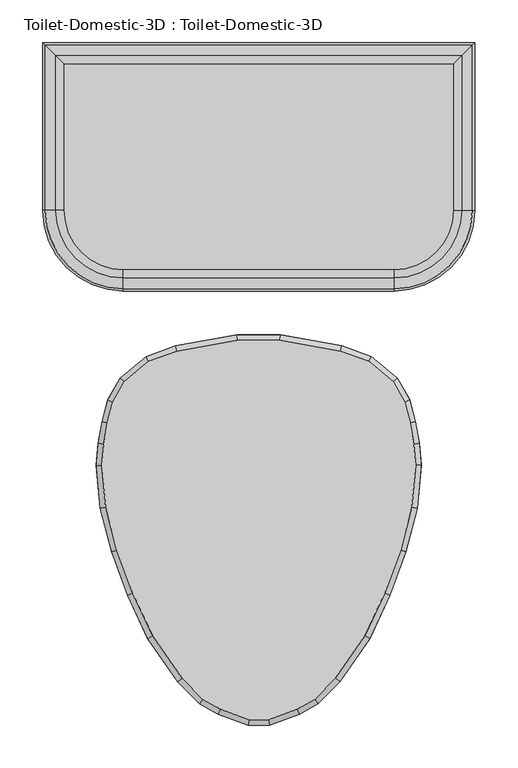
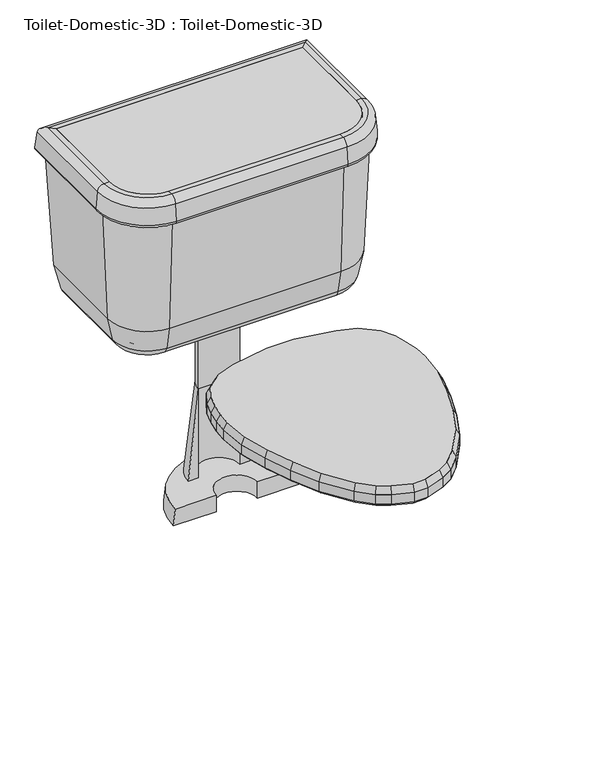
"""IFC4 building model written with IfcOpenShell, lengths in millimetres: flow terminal geometry, Toilet-Domestic-3D : Toilet-Domestic-3D."""

from ifc_helpers import new_model, si_unit, point, frame, frame_2d, origin, place, context, project, spatial, polyline, circle_curve, ellipse_curve, trimmed, segment, composite_curve, outline, extrude, faceted_brep, source, transform, mapped, element, save
from ifc_brep_helpers import plane_surface, cylinder_surface, revolved_surface, advanced_brep


def toilet_domestic_3d_toilet_domestic_3d_30431060(model_context):
    return source(origin(), model_context, "Body", "SolidModel", [
        advanced_brep(
        [(177.8, 419.1, 387.2181453), (177.8, 419.1, 374.65), (177.8, 298.45, 374.65), (177.8, 298.45, 387.2181453), (192.8020829, 434.1020829, 387.2181453), (192.8020829, 298.45, 387.2181453), (211.4650931, 452.7650931, 402.4478636), (211.4650931, 298.45, 402.4478636), (218.7732506, 460.0732506, 438.15), (218.7732506, 298.45, 438.15), (228.5868869, 469.8868869, 654.05), (228.5868869, 298.45, 654.05), (228.5868869, 469.8868869, 704.85), (228.5868869, 298.45, 704.85), (237.91817, 479.21817, 704.85), (237.91817, 298.45, 704.85), (250.5698426, 491.8698426, 693.2568779), (250.5698426, 298.45, 693.2568779), (253.3960274, 494.6960274, 660.953439), (253.3960274, 298.45, 660.953439), (247.070191, 488.370191, 654.05), (247.070191, 298.45, 654.05), (241.3, 482.6, 654.05), (241.3, 298.45, 654.05), (231.4863636, 472.7863636, 438.15), (231.4863636, 298.45, 438.15), (222.3416824, 463.6416824, 393.4759963), (222.3416824, 298.45, 393.4759963), (197.8071664, 439.1071664, 374.65), (197.8071664, 298.45, 374.65), (158.75, 279.4, 387.2181453), (158.75, 279.4, 374.65), (158.75, 264.3979171, 387.2181453), (158.75, 245.7349069, 402.4478636), (158.75, 238.4267494, 438.15), (158.75, 228.6131131, 654.05), (158.75, 228.6131131, 704.85), (158.75, 219.28183, 704.85), (158.75, 206.6301574, 693.2568779), (158.75, 203.8039726, 660.953439), (158.75, 210.129809, 654.05), (158.75, 215.9, 654.05), (158.75, 225.7136364, 438.15), (158.75, 234.8583176, 393.4759963), (158.75, 259.3928336, 374.65), (-158.75, 279.4, 374.65), (-158.75, 279.4, 387.2181453), (-158.75, 264.3979171, 387.2181453), (-158.75, 245.7349069, 402.4478636), (-158.75, 238.4267494, 438.15), (-158.75, 228.6131131, 654.05), (-158.75, 228.6131131, 704.85), (-158.75, 219.28183, 704.85), (-158.75, 206.6301574, 693.2568779), (-158.75, 203.8039726, 660.953439), (-158.75, 210.129809, 654.05), (-158.75, 215.9, 654.05), (-158.75, 225.7136364, 438.15), (-158.75, 234.8583176, 393.4759963), (-158.75, 259.3928336, 374.65), (-177.8, 298.45, 387.2181453), (-177.8, 298.45, 374.65), (-192.8020829, 298.45, 387.2181453), (-211.4650931, 298.45, 402.4478636), (-218.7732506, 298.45, 438.15), (-228.5868869, 298.45, 654.05), (-228.5868869, 298.45, 704.85), (-237.91817, 298.45, 704.85), (-250.5698426, 298.45, 693.2568779), (-253.3960274, 298.45, 660.953439), (-247.070191, 298.45, 654.05), (-241.3, 298.45, 654.05), (-231.4863636, 298.45, 438.15), (-222.3416824, 298.45, 393.4759963), (-197.8071664, 298.45, 374.65), (-177.8, 419.1, 374.65), (-177.8, 419.1, 387.2181453), (-192.8020829, 434.1020829, 387.2181453), (-211.4650931, 452.7650931, 402.4478636), (-218.7732506, 460.0732506, 438.15), (-228.5868869, 469.8868869, 654.05), (-228.5868869, 469.8868869, 704.85), (-237.91817, 479.21817, 704.85), (-250.5698426, 491.8698426, 693.2568779), (-253.3960274, 494.6960274, 660.953439), (-247.070191, 488.370191, 654.05), (-241.3, 482.6, 654.05), (-231.4863636, 472.7863636, 438.15), (-222.3416824, 463.6416824, 393.4759963), (-197.8071664, 439.1071664, 374.65)],
        [
            (0, 1),
            (1, 2),
            (2, 3),
            (3, 0),
            (4, 0),
            (3, 5),
            (5, 4),
            (6, 4, ellipse_curve(frame((192.8020829, 434.1020829, 406.2681453), z_axis=(-0.7071067811865451, 0.7071067811865498, 0.0), x_axis=(-0.7071067811865497, -0.7071067811865452, 0.0)), 26.9407684, 19.05)),
            (5, 7, circle_curve(frame((192.8020829, 298.45, 406.2681453), z_axis=(0.0, -1.0, 0.0), x_axis=(1.0, 0.0, 0.0)), 19.05)),
            (7, 6),
            (8, 6),
            (7, 9),
            (9, 8),
            (10, 8),
            (9, 11),
            (11, 10),
            (12, 10),
            (11, 13),
            (13, 12),
            (14, 12),
            (13, 15),
            (15, 14),
            (16, 14, ellipse_curve(frame((237.91817, 479.21817, 692.15), z_axis=(0.7071067811865451, -0.7071067811865498, 0.0), x_axis=(0.7071067811865497, 0.7071067811865452, 0.0)), 17.9605122, 12.7)),
            (15, 17, circle_curve(frame((237.91817, 298.45, 692.15), z_axis=(0.0, 1.0, 0.0), x_axis=(1.0, 0.0, 0.0)), 12.7)),
            (17, 16),
            (18, 16),
            (17, 19),
            (19, 18),
            (20, 18, ellipse_curve(frame((247.070191, 488.370191, 660.4), z_axis=(0.7071067811865451, -0.7071067811865498, 0.0), x_axis=(0.7071067811865497, 0.7071067811865452, 0.0)), 8.9802561, 6.35)),
            (19, 21, circle_curve(frame((247.070191, 298.45, 660.4), z_axis=(0.0, 1.0, 0.0), x_axis=(1.0, 0.0, 0.0)), 6.35)),
            (21, 20),
            (22, 20),
            (21, 23),
            (23, 22),
            (24, 22),
            (23, 25),
            (25, 24),
            (26, 24),
            (25, 27),
            (27, 26),
            (28, 26, ellipse_curve(frame((197.8071664, 439.1071664, 400.05), z_axis=(0.7071067811865451, -0.7071067811865498, 0.0), x_axis=(0.7071067811865497, 0.7071067811865452, 0.0)), 35.9210245, 25.4)),
            (27, 29, circle_curve(frame((197.8071664, 298.45, 400.05), z_axis=(0.0, 1.0, 0.0), x_axis=(1.0, 0.0, 0.0)), 25.4)),
            (29, 28),
            (1, 28),
            (29, 2),
            (30, 3, circle_curve(frame((158.75, 298.45, 387.2181453), z_axis=(0.0, 0.0, 1.0), x_axis=(1.0, 0.0, 0.0)), 19.05)),
            (2, 31, circle_curve(frame((158.75, 298.45, 374.65), z_axis=(0.0, 0.0, -1.0), x_axis=(1.0, 0.0, 0.0)), 19.05)),
            (31, 30),
            (32, 5, circle_curve(frame((158.75, 298.45, 387.2181453), z_axis=(0.0, 0.0, 1.0), x_axis=(1.0, 0.0, 0.0)), 34.0520829)),
            (30, 32),
            (33, 7, circle_curve(frame((158.75, 298.45, 402.4478636), z_axis=(0.0, 0.0, 1.0), x_axis=(1.0, 0.0, 0.0)), 52.7150931)),
            (32, 33, circle_curve(frame((158.75, 264.3979171, 406.2681453), z_axis=(-1.0, 0.0, 0.0), x_axis=(0.0, -1.0, 0.0)), 19.05)),
            (34, 9, circle_curve(frame((158.75, 298.45, 438.15), z_axis=(0.0, 0.0, 1.0), x_axis=(1.0, 0.0, 0.0)), 60.0232506)),
            (33, 34),
            (35, 11, circle_curve(frame((158.75, 298.45, 654.05), z_axis=(0.0, 0.0, 1.0), x_axis=(1.0, 0.0, 0.0)), 69.8368869)),
            (34, 35),
            (36, 13, circle_curve(frame((158.75, 298.45, 704.85), z_axis=(0.0, 0.0, 1.0), x_axis=(1.0, 0.0, 0.0)), 69.8368869)),
            (35, 36),
            (37, 15, circle_curve(frame((158.75, 298.45, 704.85), z_axis=(0.0, 0.0, 1.0), x_axis=(1.0, 0.0, 0.0)), 79.16817)),
            (36, 37),
            (38, 17, circle_curve(frame((158.75, 298.45, 693.2568779), z_axis=(0.0, 0.0, 1.0), x_axis=(1.0, 0.0, 0.0)), 91.8198426)),
            (37, 38, circle_curve(frame((158.75, 219.28183, 692.15), z_axis=(1.0, 0.0, 0.0), x_axis=(0.0, -1.0, 0.0)), 12.7)),
            (39, 19, circle_curve(frame((158.75, 298.45, 660.953439), z_axis=(0.0, 0.0, 1.0), x_axis=(1.0, 0.0, 0.0)), 94.6460274)),
            (38, 39),
            (40, 21, circle_curve(frame((158.75, 298.45, 654.05), z_axis=(0.0, 0.0, 1.0), x_axis=(1.0, 0.0, 0.0)), 88.320191)),
            (39, 40, circle_curve(frame((158.75, 210.129809, 660.4), z_axis=(1.0, 0.0, 0.0), x_axis=(0.0, -1.0, 0.0)), 6.35)),
            (41, 23, circle_curve(frame((158.75, 298.45, 654.05), z_axis=(0.0, 0.0, 1.0), x_axis=(1.0, 0.0, 0.0)), 82.55)),
            (40, 41),
            (42, 25, circle_curve(frame((158.75, 298.45, 438.15), z_axis=(0.0, 0.0, 1.0), x_axis=(1.0, 0.0, 0.0)), 72.7363636)),
            (41, 42),
            (43, 27, circle_curve(frame((158.75, 298.45, 393.4759963), z_axis=(0.0, 0.0, 1.0), x_axis=(1.0, 0.0, 0.0)), 63.5916824)),
            (42, 43),
            (44, 29, circle_curve(frame((158.75, 298.45, 374.65), z_axis=(0.0, 0.0, 1.0), x_axis=(1.0, 0.0, 0.0)), 39.0571664)),
            (43, 44, circle_curve(frame((158.75, 259.3928336, 400.05), z_axis=(1.0, 0.0, 0.0), x_axis=(0.0, -1.0, 0.0)), 25.4)),
            (44, 31),
            (31, 45),
            (45, 46),
            (46, 30),
            (46, 47),
            (47, 32),
            (47, 48, circle_curve(frame((-158.75, 264.3979171, 406.2681453), z_axis=(-1.0, 0.0, 0.0), x_axis=(0.0, -1.0, 0.0)), 19.05)),
            (48, 33),
            (48, 49),
            (49, 34),
            (49, 50),
            (50, 35),
            (50, 51),
            (51, 36),
            (51, 52),
            (52, 37),
            (52, 53, circle_curve(frame((-158.75, 219.28183, 692.15), z_axis=(1.0, 0.0, 0.0), x_axis=(0.0, -1.0, 0.0)), 12.7)),
            (53, 38),
            (53, 54),
            (54, 39),
            (54, 55, circle_curve(frame((-158.75, 210.129809, 660.4), z_axis=(1.0, 0.0, 0.0), x_axis=(0.0, -1.0, 0.0)), 6.35)),
            (55, 40),
            (55, 56),
            (56, 41),
            (56, 57),
            (57, 42),
            (57, 58),
            (58, 43),
            (58, 59, circle_curve(frame((-158.75, 259.3928336, 400.05), z_axis=(1.0, 0.0, 0.0), x_axis=(0.0, -1.0, 0.0)), 25.4)),
            (59, 44),
            (59, 45),
            (60, 46, circle_curve(frame((-158.75, 298.45, 387.2181453), z_axis=(0.0, 0.0, 1.0), x_axis=(0.0, -1.0, 0.0)), 19.05)),
            (45, 61, circle_curve(frame((-158.75, 298.45, 374.65), z_axis=(0.0, 0.0, -1.0), x_axis=(0.0, -1.0, 0.0)), 19.05)),
            (61, 60),
            (62, 47, circle_curve(frame((-158.75, 298.45, 387.2181453), z_axis=(0.0, 0.0, 1.0), x_axis=(0.0, -1.0, 0.0)), 34.0520829)),
            (60, 62),
            (63, 48, circle_curve(frame((-158.75, 298.45, 402.4478636), z_axis=(0.0, 0.0, 1.0), x_axis=(0.0, -1.0, 0.0)), 52.7150931)),
            (62, 63, circle_curve(frame((-192.8020829, 298.45, 406.2681453), z_axis=(0.0, 1.0, 0.0), x_axis=(-1.0, 0.0, 0.0)), 19.05)),
            (64, 49, circle_curve(frame((-158.75, 298.45, 438.15), z_axis=(0.0, 0.0, 1.0), x_axis=(0.0, -1.0, 0.0)), 60.0232506)),
            (63, 64),
            (65, 50, circle_curve(frame((-158.75, 298.45, 654.05), z_axis=(0.0, 0.0, 1.0), x_axis=(0.0, -1.0, 0.0)), 69.8368869)),
            (64, 65),
            (66, 51, circle_curve(frame((-158.75, 298.45, 704.85), z_axis=(0.0, 0.0, 1.0), x_axis=(0.0, -1.0, 0.0)), 69.8368869)),
            (65, 66),
            (67, 52, circle_curve(frame((-158.75, 298.45, 704.85), z_axis=(0.0, 0.0, 1.0), x_axis=(0.0, -1.0, 0.0)), 79.16817)),
            (66, 67),
            (68, 53, circle_curve(frame((-158.75, 298.45, 693.2568779), z_axis=(0.0, 0.0, 1.0), x_axis=(0.0, -1.0, 0.0)), 91.8198426)),
            (67, 68, circle_curve(frame((-237.91817, 298.45, 692.15), z_axis=(0.0, -1.0, 0.0), x_axis=(-1.0, 0.0, 0.0)), 12.7)),
            (69, 54, circle_curve(frame((-158.75, 298.45, 660.953439), z_axis=(0.0, 0.0, 1.0), x_axis=(0.0, -1.0, 0.0)), 94.6460274)),
            (68, 69),
            (70, 55, circle_curve(frame((-158.75, 298.45, 654.05), z_axis=(0.0, 0.0, 1.0), x_axis=(0.0, -1.0, 0.0)), 88.320191)),
            (69, 70, circle_curve(frame((-247.070191, 298.45, 660.4), z_axis=(0.0, -1.0, 0.0), x_axis=(-1.0, 0.0, 0.0)), 6.35)),
            (71, 56, circle_curve(frame((-158.75, 298.45, 654.05), z_axis=(0.0, 0.0, 1.0), x_axis=(0.0, -1.0, 0.0)), 82.55)),
            (70, 71),
            (72, 57, circle_curve(frame((-158.75, 298.45, 438.15), z_axis=(0.0, 0.0, 1.0), x_axis=(0.0, -1.0, 0.0)), 72.7363636)),
            (71, 72),
            (73, 58, circle_curve(frame((-158.75, 298.45, 393.4759963), z_axis=(0.0, 0.0, 1.0), x_axis=(0.0, -1.0, 0.0)), 63.5916824)),
            (72, 73),
            (74, 59, circle_curve(frame((-158.75, 298.45, 374.65), z_axis=(0.0, 0.0, 1.0), x_axis=(0.0, -1.0, 0.0)), 39.0571664)),
            (73, 74, circle_curve(frame((-197.8071664, 298.45, 400.05), z_axis=(0.0, -1.0, 0.0), x_axis=(-1.0, 0.0, 0.0)), 25.4)),
            (74, 61),
            (61, 75),
            (75, 76),
            (76, 60),
            (76, 77),
            (77, 62),
            (77, 78, ellipse_curve(frame((-192.8020829, 434.1020829, 406.2681453), z_axis=(0.7071067811865498, 0.7071067811865451, 0.0), x_axis=(-0.7071067811865451, 0.70710678118655, 0.0)), 26.9407684, 19.05)),
            (78, 63),
            (78, 79),
            (79, 64),
            (79, 80),
            (80, 65),
            (80, 81),
            (81, 66),
            (81, 82),
            (82, 67),
            (82, 83, ellipse_curve(frame((-237.91817, 479.21817, 692.15), z_axis=(-0.7071067811865498, -0.7071067811865451, 0.0), x_axis=(0.7071067811865451, -0.70710678118655, 0.0)), 17.9605122, 12.7)),
            (83, 68),
            (83, 84),
            (84, 69),
            (84, 85, ellipse_curve(frame((-247.070191, 488.370191, 660.4), z_axis=(-0.7071067811865498, -0.7071067811865451, 0.0), x_axis=(0.7071067811865451, -0.70710678118655, 0.0)), 8.9802561, 6.35)),
            (85, 70),
            (85, 86),
            (86, 71),
            (86, 87),
            (87, 72),
            (87, 88),
            (88, 73),
            (88, 89, ellipse_curve(frame((-197.8071664, 439.1071664, 400.05), z_axis=(-0.7071067811865498, -0.7071067811865451, 0.0), x_axis=(0.7071067811865451, -0.70710678118655, 0.0)), 35.9210245, 25.4)),
            (89, 74),
            (89, 75),
            (75, 1),
            (0, 76),
            (4, 77),
            (6, 78),
            (8, 79),
            (10, 80),
            (12, 81),
            (14, 82),
            (16, 83),
            (18, 84),
            (20, 85),
            (22, 86),
            (24, 87),
            (26, 88),
            (28, 89),
        ],
        [
            plane_surface(frame((177.8, 419.1, 374.65), z_axis=(-1.0, 0.0, 0.0), x_axis=(0.0, -1.0, 0.0))),
            plane_surface(frame((177.8, 419.1, 387.2181453), z_axis=(0.0, 0.0, 1.0), x_axis=(0.0, -1.0, 0.0))),
            revolved_surface(polyline([(211.8520829, 298.45, 406.2681453), (211.8520829, 453.1520829260162, 406.2681453)]), (192.8020829, 419.1, 406.2681453), (0.0, -1.0, 0.0)),
            plane_surface(frame((211.4650931, 452.7650931, 402.4478636), z_axis=(-0.9796855721787505, 0.0, 0.2005397209153197), x_axis=(0.0, -1.0, 0.0))),
            plane_surface(frame((218.7732506, 460.0732506, 438.15), z_axis=(-0.9989685402102995, 0.0, 0.045407660918654086), x_axis=(0.0, -1.0, 0.0))),
            plane_surface(frame((228.5868869, 469.8868869, 654.05), z_axis=(-1.0, 0.0, 0.0), x_axis=(0.0, -1.0, 0.0))),
            plane_surface(frame((228.5868869, 469.8868869, 704.85), z_axis=(0.0, 0.0, 1.0), x_axis=(0.0, -1.0, 0.0))),
            cylinder_surface(frame((237.91817, 419.1, 692.15), z_axis=(0.0, 1.0, 0.0), x_axis=(1.0, 0.0, 0.0)), 12.7),
            plane_surface(frame((250.5698426, 491.8698426, 693.2568779), z_axis=(0.9961946980917452, 0.0, 0.08715574274766269), x_axis=(0.0, -1.0, 0.0))),
            cylinder_surface(frame((247.070191, 419.1, 660.4), z_axis=(0.0, 1.0, 0.0), x_axis=(1.0, 0.0, 0.0)), 6.35),
            plane_surface(frame((247.070191, 488.370191, 654.05), z_axis=(0.0, 0.0, -1.0), x_axis=(0.0, -1.0, 0.0))),
            plane_surface(frame((241.3, 482.6, 654.05), z_axis=(0.9989685402102993, 0.0, -0.04540766091865594), x_axis=(0.0, -1.0, 0.0))),
            plane_surface(frame((231.4863636, 472.7863636, 438.15), z_axis=(0.9796855721787489, 0.0, -0.20053972091532798), x_axis=(0.0, -1.0, 0.0))),
            cylinder_surface(frame((197.8071664, 419.1, 400.05), z_axis=(0.0, 1.0, 0.0), x_axis=(1.0, 0.0, 0.0)), 25.4),
            plane_surface(frame((197.8071664, 439.1071664, 374.65), z_axis=(0.0, 0.0, -1.0), x_axis=(0.0, -1.0, 0.0))),
            revolved_surface(polyline([(177.8, 298.45, 374.65), (177.8, 298.45, 387.2181453)]), (158.75, 298.45, 0.0), (0.0, 0.0, -1.0)),
            plane_surface(frame((158.75, 298.45, 387.2181453), z_axis=(0.0, 0.0, 1.0), x_axis=(1.0, 0.0, 0.0))),
            revolved_surface(trimmed(ellipse_curve(frame((192.8020829, 298.45, 406.2681453), z_axis=(0.0, -1.0, 0.0), x_axis=(1.0, 0.0, 0.0)), 19.05, 19.05), [point((192.8020829, 298.45, 387.2181453))], [point((211.4650931, 298.45, 402.4478636))], True, "CARTESIAN"), (158.75, 298.45, 0.0), (0.0, 0.0, -1.0)),
            revolved_surface(polyline([(211.4650931, 298.45, 402.4478636), (218.7732506, 298.45, 438.15)]), (158.75, 298.45, 0.0), (0.0, 0.0, -1.0)),
            revolved_surface(polyline([(218.7732506, 298.45, 438.15), (228.5868869, 298.45, 654.05)]), (158.75, 298.45, 0.0), (0.0, 0.0, -1.0)),
            revolved_surface(polyline([(228.5868869, 298.45, 654.05), (228.5868869, 298.45, 704.85)]), (158.75, 298.45, 0.0), (0.0, 0.0, -1.0)),
            plane_surface(frame((158.75, 298.45, 704.85), z_axis=(0.0, 0.0, 1.0), x_axis=(1.0, 0.0, 0.0))),
            revolved_surface(trimmed(ellipse_curve(frame((237.91817, 298.45, 692.15), z_axis=(0.0, 1.0, 0.0), x_axis=(1.0, 0.0, 0.0)), 12.7, 12.7), [point((237.91817, 298.45, 704.85))], [point((250.5698426, 298.45, 693.2568779))], True, "CARTESIAN"), (158.75, 298.45, 0.0), (0.0, 0.0, -1.0)),
            revolved_surface(polyline([(250.5698426, 298.45, 693.2568779), (253.3960274, 298.45, 660.953439)]), (158.75, 298.45, 0.0), (0.0, 0.0, -1.0)),
            revolved_surface(trimmed(ellipse_curve(frame((247.070191, 298.45, 660.4), z_axis=(0.0, 1.0, 0.0), x_axis=(1.0, 0.0, 0.0)), 6.35, 6.35), [point((253.3960274, 298.45, 660.953439))], [point((247.070191, 298.45, 654.05))], True, "CARTESIAN"), (158.75, 298.45, 0.0), (0.0, 0.0, -1.0)),
            plane_surface(frame((158.75, 298.45, 654.05), z_axis=(0.0, 0.0, -1.0), x_axis=(1.0, 0.0, 0.0))),
            revolved_surface(polyline([(241.3, 298.45, 654.05), (231.4863636, 298.45, 438.15)]), (158.75, 298.45, 0.0), (0.0, 0.0, -1.0)),
            revolved_surface(polyline([(231.4863636, 298.45, 438.15), (222.3416824, 298.45, 393.4759963)]), (158.75, 298.45, 0.0), (0.0, 0.0, -1.0)),
            revolved_surface(trimmed(ellipse_curve(frame((197.8071664, 298.45, 400.05), z_axis=(0.0, 1.0, 0.0), x_axis=(1.0, 0.0, 0.0)), 25.4, 25.4), [point((222.3416824, 298.45, 393.4759963))], [point((197.8071664, 298.45, 374.65))], True, "CARTESIAN"), (158.75, 298.45, 0.0), (0.0, 0.0, -1.0)),
            plane_surface(frame((158.75, 298.45, 374.65), z_axis=(0.0, 0.0, -1.0), x_axis=(1.0, 0.0, 0.0))),
            plane_surface(frame((158.75, 279.4, 374.65), z_axis=(0.0, 1.0, 0.0), x_axis=(-1.0, 0.0, 0.0))),
            plane_surface(frame((158.75, 279.4, 387.2181453), z_axis=(0.0, 0.0, 1.0), x_axis=(-1.0, 0.0, 0.0))),
            revolved_surface(polyline([(-158.75, 245.34791709999996, 406.2681453), (158.75, 245.34791709999996, 406.2681453)]), (158.75, 264.3979171, 406.2681453), (-1.0, 0.0, 0.0)),
            plane_surface(frame((158.75, 245.7349069, 402.4478636), z_axis=(0.0, 0.9796855721787505, 0.2005397209153197), x_axis=(-1.0, 0.0, 0.0))),
            plane_surface(frame((158.75, 238.4267494, 438.15), z_axis=(0.0, 0.9989685402102995, 0.045407660918654086), x_axis=(-1.0, 0.0, 0.0))),
            plane_surface(frame((158.75, 228.6131131, 654.05), z_axis=(0.0, 1.0, 0.0), x_axis=(-1.0, 0.0, 0.0))),
            plane_surface(frame((158.75, 228.6131131, 704.85), z_axis=(0.0, 0.0, 1.0), x_axis=(-1.0, 0.0, 0.0))),
            cylinder_surface(frame((158.75, 219.28183, 692.15), z_axis=(1.0, 0.0, 0.0), x_axis=(0.0, -1.0, 0.0)), 12.7),
            plane_surface(frame((158.75, 206.6301574, 693.2568779), z_axis=(0.0, -0.9961946980917452, 0.08715574274766269), x_axis=(-1.0, 0.0, 0.0))),
            cylinder_surface(frame((158.75, 210.129809, 660.4), z_axis=(1.0, 0.0, 0.0), x_axis=(0.0, -1.0, 0.0)), 6.35),
            plane_surface(frame((158.75, 210.129809, 654.05), z_axis=(0.0, 0.0, -1.0), x_axis=(-1.0, 0.0, 0.0))),
            plane_surface(frame((158.75, 215.9, 654.05), z_axis=(0.0, -0.9989685402102993, -0.04540766091865594), x_axis=(-1.0, 0.0, 0.0))),
            plane_surface(frame((158.75, 225.7136364, 438.15), z_axis=(0.0, -0.9796855721787489, -0.20053972091532798), x_axis=(-1.0, 0.0, 0.0))),
            cylinder_surface(frame((158.75, 259.3928336, 400.05), z_axis=(1.0, 0.0, 0.0), x_axis=(0.0, -1.0, 0.0)), 25.4),
            plane_surface(frame((158.75, 259.3928336, 374.65), z_axis=(0.0, 0.0, -1.0), x_axis=(-1.0, 0.0, 0.0))),
            revolved_surface(polyline([(-158.75, 279.4, 374.65), (-158.75, 279.4, 387.2181453)]), (-158.75, 298.45, 0.0), (0.0, 0.0, -1.0)),
            plane_surface(frame((-158.75, 298.45, 387.2181453), z_axis=(0.0, 0.0, 1.0), x_axis=(0.0, -1.0, 0.0))),
            revolved_surface(trimmed(ellipse_curve(frame((-158.75, 264.3979171, 406.2681453), z_axis=(-1.0, 0.0, 0.0), x_axis=(0.0, -1.0, 0.0)), 19.05, 19.05), [point((-158.75, 264.3979171, 387.2181453))], [point((-158.75, 245.7349069, 402.4478636))], True, "CARTESIAN"), (-158.75, 298.45, 0.0), (0.0, 0.0, -1.0)),
            revolved_surface(polyline([(-158.75, 245.7349069, 402.4478636), (-158.75, 238.4267494, 438.15)]), (-158.75, 298.45, 0.0), (0.0, 0.0, -1.0)),
            revolved_surface(polyline([(-158.75, 238.4267494, 438.15), (-158.75, 228.6131131, 654.05)]), (-158.75, 298.45, 0.0), (0.0, 0.0, -1.0)),
            revolved_surface(polyline([(-158.75, 228.6131131, 654.05), (-158.75, 228.6131131, 704.85)]), (-158.75, 298.45, 0.0), (0.0, 0.0, -1.0)),
            plane_surface(frame((-158.75, 298.45, 704.85), z_axis=(0.0, 0.0, 1.0), x_axis=(0.0, -1.0, 0.0))),
            revolved_surface(trimmed(ellipse_curve(frame((-158.75, 219.28183, 692.15), z_axis=(1.0, 0.0, 0.0), x_axis=(0.0, -1.0, 0.0)), 12.7, 12.7), [point((-158.75, 219.28183, 704.85))], [point((-158.75, 206.6301574, 693.2568779))], True, "CARTESIAN"), (-158.75, 298.45, 0.0), (0.0, 0.0, -1.0)),
            revolved_surface(polyline([(-158.75, 206.6301574, 693.2568779), (-158.75, 203.8039726, 660.953439)]), (-158.75, 298.45, 0.0), (0.0, 0.0, -1.0)),
            revolved_surface(trimmed(ellipse_curve(frame((-158.75, 210.129809, 660.4), z_axis=(1.0, 0.0, 0.0), x_axis=(0.0, -1.0, 0.0)), 6.35, 6.35), [point((-158.75, 203.8039726, 660.953439))], [point((-158.75, 210.129809, 654.05))], True, "CARTESIAN"), (-158.75, 298.45, 0.0), (0.0, 0.0, -1.0)),
            plane_surface(frame((-158.75, 298.45, 654.05), z_axis=(0.0, 0.0, -1.0), x_axis=(0.0, -1.0, 0.0))),
            revolved_surface(polyline([(-158.75, 215.9, 654.05), (-158.75, 225.7136364, 438.15)]), (-158.75, 298.45, 0.0), (0.0, 0.0, -1.0)),
            revolved_surface(polyline([(-158.75, 225.7136364, 438.15), (-158.75, 234.8583176, 393.4759963)]), (-158.75, 298.45, 0.0), (0.0, 0.0, -1.0)),
            revolved_surface(trimmed(ellipse_curve(frame((-158.75, 259.3928336, 400.05), z_axis=(1.0, 0.0, 0.0), x_axis=(0.0, -1.0, 0.0)), 25.4, 25.4), [point((-158.75, 234.8583176, 393.4759963))], [point((-158.75, 259.3928336, 374.65))], True, "CARTESIAN"), (-158.75, 298.45, 0.0), (0.0, 0.0, -1.0)),
            plane_surface(frame((-158.75, 298.45, 374.65), z_axis=(0.0, 0.0, -1.0), x_axis=(0.0, -1.0, 0.0))),
            plane_surface(frame((-177.8, 298.45, 374.65), z_axis=(1.0, 0.0, 0.0), x_axis=(0.0, 1.0, 0.0))),
            plane_surface(frame((-177.8, 298.45, 387.2181453), z_axis=(0.0, 0.0, 1.0), x_axis=(0.0, 1.0, 0.0))),
            revolved_surface(polyline([(-211.8520829, 453.15208292601636, 406.2681453), (-211.8520829, 298.45, 406.2681453)]), (-192.8020829, 298.45, 406.2681453), (0.0, 1.0, 0.0)),
            plane_surface(frame((-211.4650931, 298.45, 402.4478636), z_axis=(0.9796855721787505, 0.0, 0.2005397209153197), x_axis=(0.0, 1.0, 0.0))),
            plane_surface(frame((-218.7732506, 298.45, 438.15), z_axis=(0.9989685402102995, 0.0, 0.045407660918654086), x_axis=(0.0, 1.0, 0.0))),
            plane_surface(frame((-228.5868869, 298.45, 654.05), z_axis=(1.0, 0.0, 0.0), x_axis=(0.0, 1.0, 0.0))),
            plane_surface(frame((-228.5868869, 298.45, 704.85), z_axis=(0.0, 0.0, 1.0), x_axis=(0.0, 1.0, 0.0))),
            cylinder_surface(frame((-237.91817, 298.45, 692.15), z_axis=(0.0, -1.0, 0.0), x_axis=(-1.0, 0.0, 0.0)), 12.7),
            plane_surface(frame((-250.5698426, 298.45, 693.2568779), z_axis=(-0.9961946980917452, 0.0, 0.08715574274766269), x_axis=(0.0, 1.0, 0.0))),
            cylinder_surface(frame((-247.070191, 298.45, 660.4), z_axis=(0.0, -1.0, 0.0), x_axis=(-1.0, 0.0, 0.0)), 6.35),
            plane_surface(frame((-247.070191, 298.45, 654.05), z_axis=(0.0, 0.0, -1.0), x_axis=(0.0, 1.0, 0.0))),
            plane_surface(frame((-241.3, 298.45, 654.05), z_axis=(-0.9989685402102993, 0.0, -0.04540766091865594), x_axis=(0.0, 1.0, 0.0))),
            plane_surface(frame((-231.4863636, 298.45, 438.15), z_axis=(-0.9796855721787489, 0.0, -0.20053972091532798), x_axis=(0.0, 1.0, 0.0))),
            cylinder_surface(frame((-197.8071664, 298.45, 400.05), z_axis=(0.0, -1.0, 0.0), x_axis=(-1.0, 0.0, 0.0)), 25.4),
            plane_surface(frame((-197.8071664, 298.45, 374.65), z_axis=(0.0, 0.0, -1.0), x_axis=(0.0, 1.0, 0.0))),
            plane_surface(frame((-177.8, 419.1, 374.65), z_axis=(0.0, -1.0, 0.0), x_axis=(1.0, 0.0, 0.0))),
            plane_surface(frame((-177.8, 419.1, 387.2181453), z_axis=(0.0, 0.0, 1.0), x_axis=(1.0, 0.0, 0.0))),
            revolved_surface(polyline([(211.85208292601635, 453.15208290000004, 406.2681453), (-211.85208292601618, 453.15208290000004, 406.2681453)]), (-177.8, 434.1020829, 406.2681453), (1.0, 0.0, 0.0)),
            plane_surface(frame((-211.4650931, 452.7650931, 402.4478636), z_axis=(0.0, -0.9796855721787505, 0.2005397209153197), x_axis=(1.0, 0.0, 0.0))),
            plane_surface(frame((-218.7732506, 460.0732506, 438.15), z_axis=(0.0, -0.9989685402102995, 0.045407660918654086), x_axis=(1.0, 0.0, 0.0))),
            plane_surface(frame((-228.5868869, 469.8868869, 654.05), z_axis=(0.0, -1.0, 0.0), x_axis=(1.0, 0.0, 0.0))),
            plane_surface(frame((-228.5868869, 469.8868869, 704.85), z_axis=(0.0, 0.0, 1.0), x_axis=(1.0, 0.0, 0.0))),
            cylinder_surface(frame((-177.8, 479.21817, 692.15), z_axis=(-1.0, 0.0, 0.0), x_axis=(0.0, 1.0, 0.0)), 12.7),
            plane_surface(frame((-250.5698426, 491.8698426, 693.2568779), z_axis=(0.0, 0.9961946980917452, 0.08715574274766269), x_axis=(1.0, 0.0, 0.0))),
            cylinder_surface(frame((-177.8, 488.370191, 660.4), z_axis=(-1.0, 0.0, 0.0), x_axis=(0.0, 1.0, 0.0)), 6.35),
            plane_surface(frame((-247.070191, 488.370191, 654.05), z_axis=(0.0, 0.0, -1.0), x_axis=(1.0, 0.0, 0.0))),
            plane_surface(frame((-241.3, 482.6, 654.05), z_axis=(0.0, 0.9989685402102993, -0.04540766091865594), x_axis=(1.0, 0.0, 0.0))),
            plane_surface(frame((-231.4863636, 472.7863636, 438.15), z_axis=(0.0, 0.9796855721787489, -0.20053972091532798), x_axis=(1.0, 0.0, 0.0))),
            cylinder_surface(frame((-177.8, 439.1071664, 400.05), z_axis=(-1.0, 0.0, 0.0), x_axis=(0.0, 1.0, 0.0)), 25.4),
            plane_surface(frame((-197.8071664, 439.1071664, 374.65), z_axis=(0.0, 0.0, -1.0), x_axis=(1.0, 0.0, 0.0))),
        ],
        [
            (0, [[1, 2, 3, 4]]),
            (1, [[5, -4, 6, 7]]),
            (2, [[8, -7, 9, 10]]),
            (3, [[11, -10, 12, 13]]),
            (4, [[14, -13, 15, 16]]),
            (5, [[17, -16, 18, 19]]),
            (6, [[20, -19, 21, 22]]),
            (7, [[23, -22, 24, 25]]),
            (8, [[26, -25, 27, 28]]),
            (9, [[29, -28, 30, 31]]),
            (10, [[32, -31, 33, 34]]),
            (11, [[35, -34, 36, 37]]),
            (12, [[38, -37, 39, 40]]),
            (13, [[41, -40, 42, 43]]),
            (14, [[44, -43, 45, -2]]),
            (15, [[46, -3, 47, 48]]),
            (16, [[49, -6, -46, 50]]),
            (17, [[51, -9, -49, 52]]),
            (18, [[53, -12, -51, 54]]),
            (19, [[55, -15, -53, 56]]),
            (20, [[57, -18, -55, 58]]),
            (21, [[59, -21, -57, 60]]),
            (22, [[61, -24, -59, 62]]),
            (23, [[63, -27, -61, 64]]),
            (24, [[65, -30, -63, 66]]),
            (25, [[67, -33, -65, 68]]),
            (26, [[69, -36, -67, 70]]),
            (27, [[71, -39, -69, 72]]),
            (28, [[73, -42, -71, 74]]),
            (29, [[-47, -45, -73, 75]]),
            (30, [[-48, 76, 77, 78]]),
            (31, [[-50, -78, 79, 80]]),
            (32, [[-52, -80, 81, 82]]),
            (33, [[-54, -82, 83, 84]]),
            (34, [[-56, -84, 85, 86]]),
            (35, [[-58, -86, 87, 88]]),
            (36, [[-60, -88, 89, 90]]),
            (37, [[-62, -90, 91, 92]]),
            (38, [[-64, -92, 93, 94]]),
            (39, [[-66, -94, 95, 96]]),
            (40, [[-68, -96, 97, 98]]),
            (41, [[-70, -98, 99, 100]]),
            (42, [[-72, -100, 101, 102]]),
            (43, [[-74, -102, 103, 104]]),
            (44, [[-75, -104, 105, -76]]),
            (45, [[106, -77, 107, 108]]),
            (46, [[109, -79, -106, 110]]),
            (47, [[111, -81, -109, 112]]),
            (48, [[113, -83, -111, 114]]),
            (49, [[115, -85, -113, 116]]),
            (50, [[117, -87, -115, 118]]),
            (51, [[119, -89, -117, 120]]),
            (52, [[121, -91, -119, 122]]),
            (53, [[123, -93, -121, 124]]),
            (54, [[125, -95, -123, 126]]),
            (55, [[127, -97, -125, 128]]),
            (56, [[129, -99, -127, 130]]),
            (57, [[131, -101, -129, 132]]),
            (58, [[133, -103, -131, 134]]),
            (59, [[-107, -105, -133, 135]]),
            (60, [[-108, 136, 137, 138]]),
            (61, [[-110, -138, 139, 140]]),
            (62, [[-112, -140, 141, 142]]),
            (63, [[-114, -142, 143, 144]]),
            (64, [[-116, -144, 145, 146]]),
            (65, [[-118, -146, 147, 148]]),
            (66, [[-120, -148, 149, 150]]),
            (67, [[-122, -150, 151, 152]]),
            (68, [[-124, -152, 153, 154]]),
            (69, [[-126, -154, 155, 156]]),
            (70, [[-128, -156, 157, 158]]),
            (71, [[-130, -158, 159, 160]]),
            (72, [[-132, -160, 161, 162]]),
            (73, [[-134, -162, 163, 164]]),
            (74, [[-135, -164, 165, -136]]),
            (75, [[-137, 166, -1, 167]]),
            (76, [[-139, -167, -5, 168]]),
            (77, [[-141, -168, -8, 169]]),
            (78, [[-143, -169, -11, 170]]),
            (79, [[-145, -170, -14, 171]]),
            (80, [[-147, -171, -17, 172]]),
            (81, [[-149, -172, -20, 173]]),
            (82, [[-151, -173, -23, 174]]),
            (83, [[-153, -174, -26, 175]]),
            (84, [[-155, -175, -29, 176]]),
            (85, [[-157, -176, -32, 177]]),
            (86, [[-159, -177, -35, 178]]),
            (87, [[-161, -178, -38, 179]]),
            (88, [[-163, -179, -41, 180]]),
            (89, [[-165, -180, -44, -166]]),
        ],
    ),
        extrude(outline(composite_curve([segment(trimmed(circle_curve(frame_2d((0.0, 342.9)), 38.1), [point((-38.1, 342.9))], [point((38.1, 342.9))], False, "CARTESIAN"), True, "CONTINUOUS"), segment(polyline([(38.1, 342.9), (-38.1, 342.9)]), True, "CONTINUOUS")], self_intersect=False)), frame((0.0, 0.0, 206.375), z_axis=(0.0, 0.0, 1.0), x_axis=(1.0, 0.0, 0.0)), (0.0, 0.0, 1.0), 130.175),
        extrude(outline(composite_curve([segment(polyline([(228.5868869, 469.8868869), (228.5868869, 298.45)]), True, "CONTINUOUS"), segment(trimmed(circle_curve(frame_2d((158.75, 298.45)), 69.8368869), [point((228.5868869, 298.45))], [point((158.75, 228.6131131))], False, "CARTESIAN"), True, "CONTINUOUS"), segment(polyline([(158.75, 228.6131131), (-158.75, 228.6131131)]), True, "CONTINUOUS"), segment(trimmed(circle_curve(frame_2d((-158.75, 298.45)), 69.8368869), [point((-158.75, 228.6131131))], [point((-228.5868869, 298.45))], False, "CARTESIAN"), True, "CONTINUOUS"), segment(polyline([(-228.5868869, 298.45), (-228.5868869, 469.8868869), (228.5868869, 469.8868869)]), True, "CONTINUOUS")], self_intersect=False)), frame((0.0, 0.0, 654.05), z_axis=(0.0, 0.0, 1.0), x_axis=(1.0, 0.0, 0.0)), (0.0, 0.0, 1.0), 50.8),
        faceted_brep([(-157.6293435, 97.472128, 400.05), (-171.060664, 73.773864, 400.05), (-177.5851102, 49.4242991, 400.05), (-181.9845715, 24.4737144, 400.05), (-184.125744, 0.0, 400.05), (-179.7950716, -49.4998127, 400.05), (-166.347, -99.688699, 400.05), (-148.0469602, -149.9676451, 400.05), (-124.7045808, -200.0255393, 400.05), (-90.0971582, -249.9125941, 400.05), (-65.691017, -274.3187354, 400.05), (-44.8990862, -286.3229622, 400.05), (-11.5803237, -298.45, 400.05), (11.5803237, -298.45, 400.05), (44.8990862, -286.3229622, 400.05), (65.691017, -274.3187354, 400.05), (90.0971582, -249.9125941, 400.05), (124.7045808, -200.0255393, 400.05), (148.0469602, -149.9676451, 400.05), (166.347, -99.688699, 400.05), (179.7950716, -49.4998127, 400.05), (184.125744, 0.0, 400.05), (181.9845715, 24.4737144, 400.05), (177.5851102, 49.4242991, 400.05), (171.060664, 73.773864, 400.05), (157.6293435, 97.472128, 400.05), (129.0942628, 121.4159037, 400.05), (95.7755003, 133.5429415, 400.05), (24.844447, 146.05, 400.05), (-24.844447, 146.05, 400.05), (-95.7755003, 133.5429415, 400.05), (-129.0942628, 121.4159037, 400.05), (-162.5887836, 101.6, 387.2181453), (-132.3182423, 127.0, 387.2181453), (-97.4252791, 139.7, 387.2181453), (-25.4, 152.4, 387.2181453), (25.4, 152.4, 387.2181453), (97.4252791, 139.7, 387.2181453), (132.3182423, 127.0, 387.2181453), (162.5887836, 101.6, 387.2181453), (176.9845865, 76.2, 387.2181453), (183.790496, 50.8, 387.2181453), (188.2862441, 25.3033453, 387.2181453), (190.5, 0.0, 387.2181453), (186.0724883, -50.6066907, 387.2181453), (172.4088722, -101.6, 387.2181453), (153.9191843, -152.4, 387.2181453), (130.2307553, -203.2, 387.2181453), (94.9900085, -254.0, 387.2181453), (69.5900085, -279.4, 387.2181453), (47.5929632, -292.1, 387.2181453), (12.7, -304.8, 387.2181453), (-12.7, -304.8, 387.2181453), (-47.5929632, -292.1, 387.2181453), (-69.5900085, -279.4, 387.2181453), (-94.9900085, -254.0, 387.2181453), (-130.2307553, -203.2, 387.2181453), (-153.9191843, -152.4, 387.2181453), (-172.4088722, -101.6, 387.2181453), (-186.0724883, -50.6066907, 387.2181453), (-190.5, 0.0, 387.2181453), (-188.2862441, 25.3033453, 387.2181453), (-183.790496, 50.8, 387.2181453), (-176.9845865, 76.2, 387.2181453)], [[[0, 1, 2, 3, 4, 5, 6, 7, 8, 9, 10, 11, 12, 13, 14, 15, 16, 17, 18, 19, 20, 21, 22, 23, 24, 25, 26, 27, 28, 29, 30, 31]], [[32, 33, 34, 35, 36, 37, 38, 39, 40, 41, 42, 43, 44, 45, 46, 47, 48, 49, 50, 51, 52, 53, 54, 55, 56, 57, 58, 59, 60, 61, 62, 63]], [[32, 63, 1, 0]], [[63, 62, 2, 1]], [[62, 61, 3, 2]], [[61, 60, 4, 3]], [[60, 59, 5, 4]], [[59, 58, 6, 5]], [[58, 57, 7, 6]], [[57, 56, 8, 7]], [[56, 55, 9, 8]], [[55, 54, 10, 9]], [[54, 53, 11, 10]], [[53, 52, 12, 11]], [[52, 51, 13, 12]], [[51, 50, 14, 13]], [[50, 49, 15, 14]], [[49, 48, 16, 15]], [[48, 47, 17, 16]], [[47, 46, 18, 17]], [[46, 45, 19, 18]], [[45, 44, 20, 19]], [[44, 43, 21, 20]], [[43, 42, 22, 21]], [[42, 41, 23, 22]], [[41, 40, 24, 23]], [[40, 39, 25, 24]], [[39, 38, 26, 25]], [[38, 37, 27, 26]], [[37, 36, 28, 27]], [[36, 35, 29, 28]], [[35, 34, 30, 29]], [[34, 33, 31, 30]], [[33, 32, 0, 31]]]),
        advanced_brep(
        [(-38.1, 342.9, 206.375), (-57.15, 342.9, 31.75), (-38.1, 342.9, 31.75), (38.1, 342.9, 206.375), (38.1, 342.9, 31.75), (57.15, 342.9, 31.75)],
        [
            (0, 1),
            (1, 2),
            (2, 0),
            (3, 4),
            (4, 5),
            (5, 3),
            (5, 1, circle_curve(frame((0.0, 342.9, 31.75), z_axis=(0.0, 0.0, 1.0), x_axis=(-1.0, 0.0, 0.0)), 57.15)),
            (0, 3, circle_curve(frame((0.0, 342.9, 206.375), z_axis=(0.0, 0.0, -1.0), x_axis=(-1.0, 0.0, 0.0)), 38.1)),
            (4, 2, circle_curve(frame((0.0, 342.9, 31.75), z_axis=(0.0, 0.0, 1.0), x_axis=(-1.0, 0.0, 0.0)), 38.1)),
        ],
        [
            plane_surface(frame((0.0, 342.9, 31.75), z_axis=(0.0, -1.0, 0.0), x_axis=(-1.0, 0.0, 0.0))),
            plane_surface(frame((0.0, 342.9, 31.75), z_axis=(0.0, -1.0, 0.0), x_axis=(1.0, 0.0, 0.0))),
            revolved_surface(polyline([(-38.1, 342.9, 206.375), (-57.15, 342.9, 31.75)]), (0.0, 342.9, 31.75), (0.0, 0.0, -1.0)),
            plane_surface(frame((0.0, 342.9, 31.75), z_axis=(0.0, 0.0, -1.0), x_axis=(-1.0, 0.0, 0.0))),
            revolved_surface(polyline([(-38.1, 342.9, 31.75), (-38.1, 342.9, 206.375)]), (0.0, 342.9, 31.75), (0.0, 0.0, -1.0)),
        ],
        [
            (0, [[1, 2, 3]]),
            (1, [[4, 5, 6]]),
            (2, [[7, -1, 8, -6]]),
            (3, [[9, -2, -7, -5]]),
            (4, [[-8, -3, -9, -4]]),
        ],
    ),
        advanced_brep(
        [(-117.7636364, 285.75, 0.0), (-38.1, 285.75, 0.0), (-38.1, 285.75, 31.75), (-114.3, 285.75, 31.75), (117.7636364, 285.75, 0.0), (114.3, 285.75, 31.75), (38.1, 285.75, 31.75), (38.1, 285.75, 0.0)],
        [
            (0, 1),
            (1, 2),
            (2, 3),
            (3, 0),
            (4, 5),
            (5, 6),
            (6, 7),
            (7, 4),
            (7, 1, circle_curve(frame((0.0, 285.75, 0.0), z_axis=(0.0, 0.0, 1.0), x_axis=(-1.0, 0.0, 0.0)), 38.1)),
            (0, 4, circle_curve(frame((0.0, 285.75, 0.0), z_axis=(0.0, 0.0, -1.0), x_axis=(-1.0, 0.0, 0.0)), 117.7636364)),
            (6, 2, circle_curve(frame((0.0, 285.75, 31.75), z_axis=(0.0, 0.0, 1.0), x_axis=(-1.0, 0.0, 0.0)), 38.1)),
            (5, 3, circle_curve(frame((0.0, 285.75, 31.75), z_axis=(0.0, 0.0, 1.0), x_axis=(-1.0, 0.0, 0.0)), 114.3)),
        ],
        [
            plane_surface(frame((0.0, 285.75, -304.8), z_axis=(0.0, -1.0, 0.0), x_axis=(-1.0, 0.0, 0.0))),
            plane_surface(frame((0.0, 285.75, -304.8), z_axis=(0.0, -1.0, 0.0), x_axis=(1.0, 0.0, 0.0))),
            plane_surface(frame((0.0, 285.75, 0.0), z_axis=(0.0, 0.0, -1.0), x_axis=(-1.0, 0.0, 0.0))),
            revolved_surface(polyline([(-38.1, 285.75, 0.0), (-38.1, 285.75, 31.75)]), (0.0, 285.75, -304.8), (0.0, 0.0, -1.0)),
            plane_surface(frame((0.0, 285.75, 31.75), z_axis=(0.0, 0.0, 1.0), x_axis=(-1.0, 0.0, 0.0))),
            revolved_surface(polyline([(-114.3, 285.75, 31.75), (-117.7636364, 285.75, 0.0)]), (0.0, 285.75, -304.8), (0.0, 0.0, -1.0)),
        ],
        [
            (0, [[1, 2, 3, 4]]),
            (1, [[5, 6, 7, 8]]),
            (2, [[9, -1, 10, -8]]),
            (3, [[11, -2, -9, -7]]),
            (4, [[12, -3, -11, -6]]),
            (5, [[-10, -4, -12, -5]]),
        ],
    ),
        extrude(outline(composite_curve([segment(polyline([(177.8, 419.1), (177.8, 298.45)]), True, "CONTINUOUS"), segment(trimmed(circle_curve(frame_2d((158.75, 298.45)), 19.05), [point((177.8, 298.45))], [point((158.75, 279.4))], False, "CARTESIAN"), True, "CONTINUOUS"), segment(polyline([(158.75, 279.4), (-158.75, 279.4)]), True, "CONTINUOUS"), segment(trimmed(circle_curve(frame_2d((-158.75, 298.45)), 19.05), [point((-158.75, 279.4))], [point((-177.8, 298.45))], False, "CARTESIAN"), True, "CONTINUOUS"), segment(polyline([(-177.8, 298.45), (-177.8, 419.1), (177.8, 419.1)]), True, "CONTINUOUS")], self_intersect=False)), frame((0.0, 0.0, 374.65), z_axis=(0.0, 0.0, 1.0), x_axis=(1.0, 0.0, 0.0)), (0.0, 0.0, 1.0), 12.5681453),
        faceted_brep([(-97.4252791, 139.7, 368.3), (-132.3182423, 127.0, 368.3), (-162.5887836, 101.6, 368.3), (-176.9845865, 76.2, 368.3), (-183.790496, 50.8, 368.3), (-188.2862441, 25.3033453, 368.3), (-190.5, 0.0, 368.3), (-186.0724883, -50.6066907, 368.3), (-172.4088722, -101.6, 368.3), (-153.9191843, -152.4, 368.3), (-130.2307553, -203.2, 368.3), (-94.9900085, -254.0, 368.3), (-69.5900085, -279.4, 368.3), (-47.5929632, -292.1, 368.3), (-12.7, -304.8, 368.3), (12.7, -304.8, 368.3), (47.5929632, -292.1, 368.3), (69.5900085, -279.4, 368.3), (94.9900085, -254.0, 368.3), (130.2307553, -203.2, 368.3), (153.9191843, -152.4, 368.3), (172.4088722, -101.6, 368.3), (186.0724883, -50.6066907, 368.3), (190.5, 0.0, 368.3), (188.2862441, 25.3033453, 368.3), (183.790496, 50.8, 368.3), (176.9845865, 76.2, 368.3), (162.5887836, 101.6, 368.3), (132.3182423, 127.0, 368.3), (97.4252791, 139.7, 368.3), (25.4, 152.4, 368.3), (-25.4, 152.4, 368.3), (-95.7755003, 133.5429415, 361.95), (-24.844447, 146.05, 361.95), (24.844447, 146.05, 361.95), (95.7755003, 133.5429415, 361.95), (129.0942628, 121.4159037, 361.95), (157.6293435, 97.472128, 361.95), (171.060664, 73.773864, 361.95), (177.5851102, 49.4242991, 361.95), (181.9845715, 24.4737144, 361.95), (184.125744, 0.0, 361.95), (179.7950716, -49.4998127, 361.95), (166.347, -99.688699, 361.95), (148.0469602, -149.9676451, 361.95), (124.7045808, -200.0255393, 361.95), (90.0971582, -249.9125941, 361.95), (65.691017, -274.3187354, 361.95), (44.8990862, -286.3229622, 361.95), (11.5803237, -298.45, 361.95), (-11.5803237, -298.45, 361.95), (-44.8990862, -286.3229622, 361.95), (-65.691017, -274.3187354, 361.95), (-90.0971582, -249.9125941, 361.95), (-124.7045808, -200.0255393, 361.95), (-148.0469602, -149.9676451, 361.95), (-166.347, -99.688699, 361.95), (-179.7950716, -49.4998127, 361.95), (-184.125744, 0.0, 361.95), (-181.9845715, 24.4737144, 361.95), (-177.5851102, 49.4242991, 361.95), (-171.060664, 73.773864, 361.95), (-157.6293435, 97.472128, 361.95), (-129.0942628, 121.4159037, 361.95)], [[[0, 1, 2, 3, 4, 5, 6, 7, 8, 9, 10, 11, 12, 13, 14, 15, 16, 17, 18, 19, 20, 21, 22, 23, 24, 25, 26, 27, 28, 29, 30, 31]], [[32, 33, 34, 35, 36, 37, 38, 39, 40, 41, 42, 43, 44, 45, 46, 47, 48, 49, 50, 51, 52, 53, 54, 55, 56, 57, 58, 59, 60, 61, 62, 63]], [[32, 63, 1, 0]], [[63, 62, 2, 1]], [[62, 61, 3, 2]], [[61, 60, 4, 3]], [[60, 59, 5, 4]], [[59, 58, 6, 5]], [[58, 57, 7, 6]], [[57, 56, 8, 7]], [[56, 55, 9, 8]], [[55, 54, 10, 9]], [[54, 53, 11, 10]], [[53, 52, 12, 11]], [[52, 51, 13, 12]], [[51, 50, 14, 13]], [[50, 49, 15, 14]], [[49, 48, 16, 15]], [[48, 47, 17, 16]], [[47, 46, 18, 17]], [[46, 45, 19, 18]], [[45, 44, 20, 19]], [[44, 43, 21, 20]], [[43, 42, 22, 21]], [[42, 41, 23, 22]], [[41, 40, 24, 23]], [[40, 39, 25, 24]], [[39, 38, 26, 25]], [[38, 37, 27, 26]], [[37, 36, 28, 27]], [[36, 35, 29, 28]], [[35, 34, 30, 29]], [[34, 33, 31, 30]], [[33, 32, 0, 31]]]),
        extrude(outline(polyline([(-162.5887836, 101.6), (-132.3182423, 127.0), (-97.4252791, 139.7), (-25.4, 152.4), (25.4, 152.4), (97.4252791, 139.7), (132.3182423, 127.0), (162.5887836, 101.6), (176.9845865, 76.2), (183.790496, 50.8), (188.2862441, 25.3033453), (190.5, 0.0), (186.0724883, -50.6066907), (172.4088722, -101.6), (153.9191843, -152.4), (130.2307553, -203.2), (94.9900085, -254.0), (69.5900085, -279.4), (47.5929632, -292.1), (12.7, -304.8), (-12.7, -304.8), (-47.5929632, -292.1), (-69.5900085, -279.4), (-94.9900085, -254.0), (-130.2307553, -203.2), (-153.9191843, -152.4), (-172.4088722, -101.6), (-186.0724883, -50.6066907), (-190.5, 0.0), (-188.2862441, 25.3033453), (-183.790496, 50.8), (-176.9845865, 76.2), (-162.5887836, 101.6)])), frame((0.0, 0.0, 368.3), z_axis=(0.0, 0.0, 1.0), x_axis=(1.0, 0.0, 0.0)), (0.0, 0.0, 1.0), 19.05),
    ])


if __name__ == "__main__":
    model = new_model("IFC4")
    model_context = context("Model", 3, world=origin())
    ifc_project = project(units=[si_unit("LENGTHUNIT", "METRE", prefix="MILLI")], contexts=[model_context])
    site = spatial("IfcSite", under=ifc_project)
    building = spatial("IfcBuilding", under=site)
    placement = place(None, origin())
    toilet_domestic_3d_toilet_domestic_3d_shape = toilet_domestic_3d_toilet_domestic_3d_30431060(model_context)
    element("IfcFlowTerminal", 1, ObjectType="Toilet-Domestic-3D : Toilet-Domestic-3D", at=placement, inside=building, context=model_context, shape_type="MappedRepresentation", body=[
        mapped(toilet_domestic_3d_toilet_domestic_3d_shape, transform((0.0, 0.0, 0.0), x_axis=(1.0, 0.0, 0.0), y_axis=(0.0, 1.0, 0.0), z_axis=(0.0, 0.0, 1.0))),
    ])
    save(model, "model.ifc")

# Revit data of these elements
# Type "Toilet-Domestic-3D : Toilet-Domestic-3D"
#   Assembly Code = "D2010110"
#   Toilet - Bowl/Basin Material = Porcelain, Linen
#   Toilet - Seat Material = Laminate, Linen, Matte
#   Default Elevation = 0
# Element 1 (IfcFlowTerminal, "Toilet-Domestic-3D : Toilet-Domestic-3D")
#   Materials on its faces: "Porcelain, Linen", "Laminate, Linen, Matte"
# Materials
#   "Porcelain, Linen": class "Ceramic", colour RGB 249 239 230, transparency 0, Description = "Porcelain, linen", Cost = 0
#   "Laminate, Linen, Matte": class "Plastic", colour RGB 249 239 230, transparency 0, Description = "Plastic Laminate - Linen, Matte", Cost = 0
